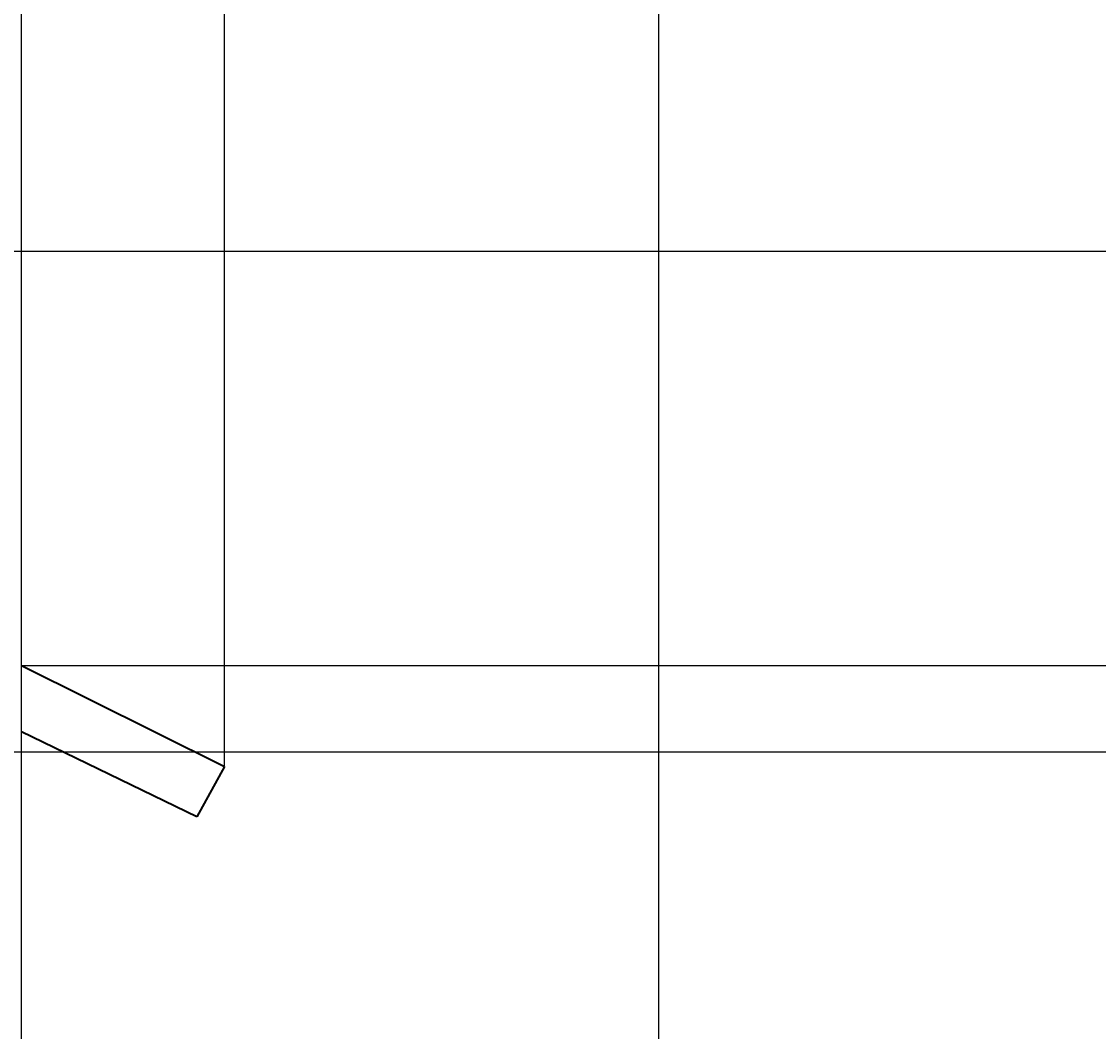
# Model space of a CAD drawing. Units: inches. Extents: x -26 to 776, y -22 to 650.
# Tile 60 of 62: x 426 to 544, y 415 to 526. Entities that reach past the tile are written whole.
import ezdxf

# ---------------------------------------------------------------- set-up
doc = ezdxf.new("R2010")
doc.units = ezdxf.units.IN
doc.header["$MEASUREMENT"] = 0
doc.layers.add('A-ANNO-DIMS', color=2, linetype='Continuous', lineweight=18)
doc.layers.add('A-ROOF', color=7, linetype='Continuous', lineweight=35)
doc.styles.get("Standard").update_dxf_attribs({"font": 'arial.ttf'})
doc.dimstyles.get("Standard").update_dxf_attribs({"dimtxt": 0.5625, "dimasz": 0.18, "dimexe": 0.18, "dimexo": 0.0625, "dimgap": 0.09, "dimtad": 0, "dimtih": 1, "dimtoh": 1, "dimdec": 4, "dimzin": 0, "dimdsep": 46, "dimlunit": 4, "dimtxsty": 'Standard', "dimcen": 0.09, "dimadec": 0, "dimazin": 0, "dimtfac": 1, "dimtdec": 4, "dimtofl": 0, "dimtmove": 0, "dimatfit": 3, "dimfxl": 1, "dimtolj": 1, "dimtzin": 0, "dimarcsym": 0})

# ---------------------------------------------------------------- blocks, each defined once
blk = doc.blocks.new('*D20')
at = {"layer": 'A-ANNO-DIMS', "color": 0, "lineweight": -2, "transparency": 16777216}
for p, q in [((425.81, 455.47), (775.34, 455.47)), ((775.16, 455.29), (775.16, 235.85)), ((775.16, 15.66), (775.16, 235.1)), ((425.81, 15.48), (775.34, 15.48))]:
    blk.add_line(p, q, dxfattribs=at)
at = {"layer": 'A-ANNO-DIMS', "color": 0, "transparency": 16777216}
for points in [[(775.13, 455.29), (775.19, 455.29), (775.16, 455.47)], [(775.13, 15.66), (775.19, 15.66), (775.16, 15.48)]]:
    blk.add_solid(points, dxfattribs=at)
at = {"layer": 'Defpoints', "color": 0, "transparency": 16777216}
for p in [(425.74, 455.47), (775.16, 455.47), (425.74, 15.48)]:
    blk.add_point(p, dxfattribs=at)
at = {"layer": 'A-ANNO-DIMS', "color": 0, "transparency": 16777216, "insert": (775.16, 235.48), "char_height": 0.562, "attachment_point": 5}
blk.add_mtext('\\A1;440', dxfattribs=at)
blk = doc.blocks.new('*D21')
at = {"layer": 'A-ANNO-DIMS', "color": 0, "lineweight": -2, "transparency": 16777216}
for p, q in [((425.74, 455.53), (425.74, 649.86)), ((425.92, 649.68), (435.83, 649.68)), ((447.83, 649.68), (437.92, 649.68)), ((448.01, 444.45), (448.01, 649.86))]:
    blk.add_line(p, q, dxfattribs=at)
at = {"layer": 'A-ANNO-DIMS', "color": 0, "transparency": 16777216}
for points in [[(425.92, 649.71), (425.92, 649.65), (425.74, 649.68)], [(447.83, 649.71), (447.83, 649.65), (448.01, 649.68)]]:
    blk.add_solid(points, dxfattribs=at)
at = {"layer": 'Defpoints', "color": 0, "transparency": 16777216}
for p in [(448.01, 649.68), (425.74, 455.47), (448.01, 444.39)]:
    blk.add_point(p, dxfattribs=at)
at = {"layer": 'A-ANNO-DIMS', "color": 0, "transparency": 16777216, "insert": (436.88, 649.68), "char_height": 0.562, "attachment_point": 5}
blk.add_mtext('\\A1;22.27', dxfattribs=at)
blk = doc.blocks.new('*D31')
at = {"layer": 'A-ANNO-DIMS', "color": 0, "lineweight": -2, "transparency": 16777216}
for p, q in [((289.3, 500.9), (775.34, 500.9)), ((775.16, 500.72), (775.16, 473.83)), ((775.16, 446.19), (775.16, 473.07)), ((285.08, 446.01), (775.34, 446.01))]:
    blk.add_line(p, q, dxfattribs=at)
at = {"layer": 'A-ANNO-DIMS', "color": 0, "transparency": 16777216}
for points in [[(775.13, 500.72), (775.19, 500.72), (775.16, 500.9)], [(775.13, 446.19), (775.19, 446.19), (775.16, 446.01)]]:
    blk.add_solid(points, dxfattribs=at)
at = {"layer": 'Defpoints', "color": 0, "transparency": 16777216}
for p in [(289.24, 500.9), (775.16, 500.9), (285.02, 446.01)]:
    blk.add_point(p, dxfattribs=at)
at = {"layer": 'A-ANNO-DIMS', "color": 0, "transparency": 16777216, "insert": (775.16, 473.45), "char_height": 0.562, "attachment_point": 5}
blk.add_mtext('\\A1;54.89', dxfattribs=at)
blk = doc.blocks.new('*D39')
at = {"layer": 'A-ANNO-DIMS', "color": 0, "lineweight": -2, "transparency": 16777216}
for p, q in [((289.24, 15.54), (289.24, 649.86)), ((289.42, 649.68), (356.48, 649.68)), ((425.56, 649.68), (358.51, 649.68)), ((425.74, 15.54), (425.74, 649.86))]:
    blk.add_line(p, q, dxfattribs=at)
at = {"layer": 'A-ANNO-DIMS', "color": 0, "transparency": 16777216}
for points in [[(289.42, 649.71), (289.42, 649.65), (289.24, 649.68)], [(425.56, 649.71), (425.56, 649.65), (425.74, 649.68)]]:
    blk.add_solid(points, dxfattribs=at)
at = {"layer": 'Defpoints', "color": 0, "transparency": 16777216}
for p in [(425.74, 649.68), (289.24, 15.48), (425.74, 15.48)]:
    blk.add_point(p, dxfattribs=at)
at = {"layer": 'A-ANNO-DIMS', "color": 0, "transparency": 16777216, "insert": (357.49, 649.68), "char_height": 0.562, "attachment_point": 5}
blk.add_mtext('\\A1;136.5', dxfattribs=at)
blk = doc.blocks.new('*D40')
at = {"layer": 'A-ANNO-DIMS', "color": 0, "lineweight": -2, "transparency": 16777216}
for p, q in [((425.74, 15.54), (425.74, 649.86)), ((425.92, 649.68), (459.65, 649.68)), ((495.45, 649.68), (461.73, 649.68)), ((495.63, 15.54), (495.63, 649.86))]:
    blk.add_line(p, q, dxfattribs=at)
at = {"layer": 'A-ANNO-DIMS', "color": 0, "transparency": 16777216}
for points in [[(425.92, 649.71), (425.92, 649.65), (425.74, 649.68)], [(495.45, 649.71), (495.45, 649.65), (495.63, 649.68)]]:
    blk.add_solid(points, dxfattribs=at)
at = {"layer": 'Defpoints', "color": 0, "transparency": 16777216}
for p in [(495.63, 649.68), (425.74, 15.48), (495.63, 15.48)]:
    blk.add_point(p, dxfattribs=at)
at = {"layer": 'A-ANNO-DIMS', "color": 0, "transparency": 16777216, "insert": (460.69, 649.68), "char_height": 0.562, "attachment_point": 5}
blk.add_mtext('\\A1;69.89', dxfattribs=at)

msp = doc.modelspace()

# ---------------------------------------------------------------- linework, layer by layer
at = {"layer": 'A-ROOF'}
for p, q in [((425.7434, 455.4717), (448.0125, 444.3909)), ((444.9683, 438.8738), (425.7434, 448.2114)), ((448.0125, 444.3909), (444.9683, 438.8738))]:
    msp.add_line(p, q, dxfattribs=at)

# ---------------------------------------------------------------- dimensions: what is measured, and where the dimension line sits
at = {"layer": 'A-ANNO-DIMS'}
for base, p1, p2, override, picture, middle in [((425.7434, 649.6763), (289.2424, 15.4824), (425.7434, 15.4824), {"dimdec": 1, "dimlfac": 1, "dimrnd": 0, "dimzin": 0, "dimdsep": 46, "dimlunit": 2}, '*D39', (357.4929, 649.6763)), ((448.0125, 649.6763), (425.7434, 455.4717), (448.0125, 444.3909), {"dimdec": 2, "dimlfac": 1, "dimrnd": 0, "dimzin": 0, "dimdsep": 46, "dimlunit": 2}, '*D21', (436.878, 649.6763)), ((495.6309, 649.6763), (425.7434, 15.4824), (495.6309, 15.4824), {"dimdec": 2, "dimlfac": 1, "dimrnd": 0, "dimzin": 0, "dimdsep": 46, "dimlunit": 2}, '*D40', (460.6872, 649.6763))]:
    dim = msp.add_linear_dim(base=base, p1=p1, p2=p2, dimstyle='Standard', override=override, dxfattribs=at)
    dim.commit()
    dim.dimension.update_dxf_attribs({"geometry": picture, "text_midpoint": middle})
for base, p1, p2, override, picture, middle in [((775.1553, 500.896), (285.0179, 446.0063), (289.2424, 500.896), {"dimdec": 2, "dimlfac": 1, "dimrnd": 0, "dimzin": 0, "dimdsep": 46, "dimlunit": 2}, '*D31', (775.1553, 473.4511)), ((775.1553, 455.4717), (425.7434, 15.4824), (425.7434, 455.4717), {"dimdec": 0, "dimlfac": 1, "dimrnd": 0, "dimzin": 0, "dimdsep": 46, "dimlunit": 2}, '*D20', (775.1553, 235.477))]:
    dim = msp.add_linear_dim(base=base, p1=p1, p2=p2, angle=90, dimstyle='Standard', override=override, dxfattribs=at)
    dim.commit()
    dim.dimension.update_dxf_attribs({"geometry": picture, "text_midpoint": middle})

doc.saveas('drawing.dxf')
